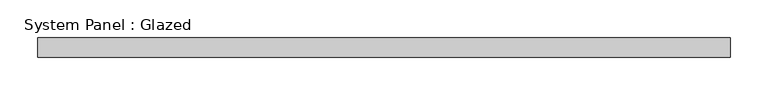
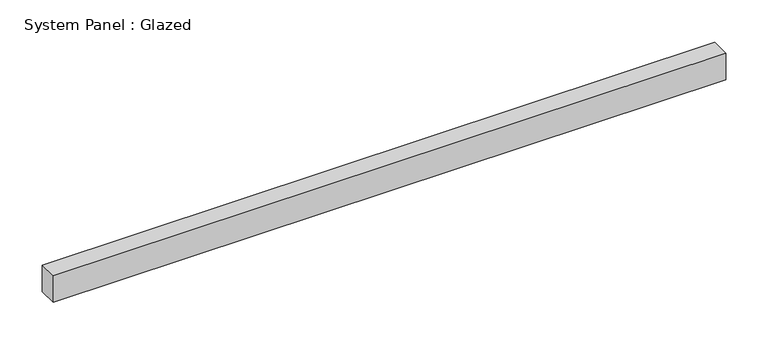
"""IFC4 building model written with IfcOpenShell, lengths in millimetres: plate geometry, System Panel : Glazed."""

from ifc_helpers import new_model, si_unit, origin, origin_with_axes, place, context, project, spatial, polyline, outline, extrude, source, transform, mapped, element, save


def system_panel_glazed_8073c085(model_context):
    return source(origin(), model_context, "Body", "SweptSolid", [
        extrude(outline(polyline([(457.2, 19.05), (-457.2, 19.05), (-457.2, 44.45), (457.2, 44.45), (457.2, 19.05)])), origin_with_axes(), (0.0, 0.0, 1.0), 38.1),
    ])


if __name__ == "__main__":
    model = new_model("IFC4")
    model_context = context("Model", 3, world=origin())
    ifc_project = project(units=[si_unit("LENGTHUNIT", "METRE", prefix="MILLI")], contexts=[model_context])
    site = spatial("IfcSite", under=ifc_project)
    building = spatial("IfcBuilding", under=site)
    placement = place(None, origin())
    system_panel_glazed_shape = system_panel_glazed_8073c085(model_context)
    element("IfcPlate", 1, ObjectType="System Panel : Glazed", at=placement, inside=building, context=model_context, shape_type="MappedRepresentation", body=[
        mapped(system_panel_glazed_shape, transform((0.0, 0.0, 0.0), x_axis=(1.0, 0.0, 0.0), y_axis=(0.0, 1.0, 0.0), z_axis=(0.0, 0.0, 1.0))),
    ])
    save(model, "model.ifc")

# Revit data of these elements
# Type "System Panel : Glazed"
#   Construction Type Id = "GSP4R"
#   Analytic Construction = "1/8 in Pilkington single glazing"
#   Visual Light Transmittance = 0.9
#   Solar Heat Gain Coefficient = 0.86
#   Heat Transfer Coefficient (U) = 1.18115 BTU/(h·ft²·°F)
# Element 1 (IfcPlate, "System Panel : Glazed")
#   Materials on its faces: "Glass"
# Materials
#   "Glass": class "Glass", colour RGB 0 128 192, transparency 0.75, Description = "Soda Lime Glass", Cost = 0
